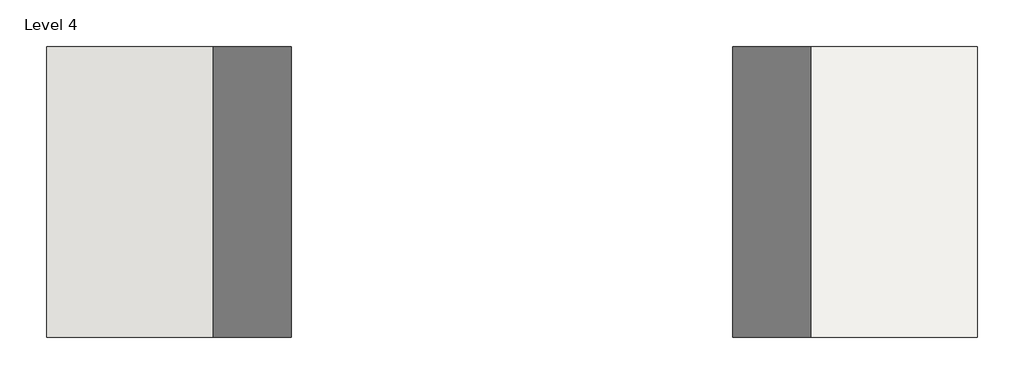
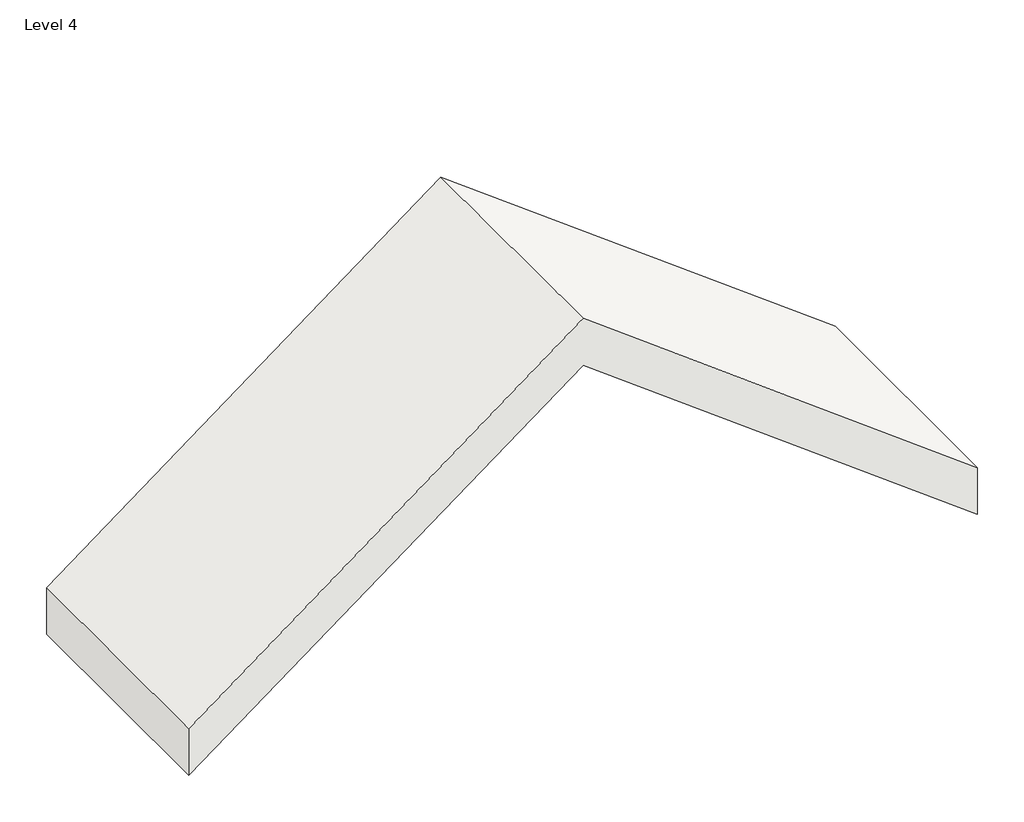
# One storey: 1 roof.
"""IFC4 building model written with IfcOpenShell, lengths in millimetres."""

from ifc_helpers import new_model, si_unit, frame, origin, place, context, project, spatial, polyline, outline, extrude, element, save

model = new_model("IFC4")

# Units and contexts
model_context = context("Model", 3, world=origin())
ifc_project = project(units=[si_unit("LENGTHUNIT", "METRE", prefix="MILLI")], contexts=[model_context])

# Site, building, storey
site = spatial("IfcSite", under=ifc_project)
building = spatial("IfcBuilding", under=site)
storey = spatial("IfcBuildingStorey", under=building, Name="Level 4", Elevation=9144.0)

# Roof
placement = place(None, origin())
element("IfcRoof", 1, ObjectType="Generic - 12\"", at=placement, inside=storey, context=model_context, shape_type="SweptSolid", body=[
    extrude(outline(polyline([(9525.0, -10404.6498106), (11809.2644938, -13450.3358024), (9525.0, -16496.0217941), (9144.0, -16496.0217941), (11428.2644938, -13450.3358024), (9144.0, -10404.6498106), (9525.0, -10404.6498106)])), frame((0.0, -12865.0511954, 0.0), z_axis=(0.0, 1.0, 0.0), x_axis=(0.0, 0.0, 1.0)), (0.0, 0.0, 1.0), 1901.825),
])

save(model, "model.ifc")

# Revit data of these elements
# Type "Generic - 12\""
#   Assembly Code = "B1020"
#   Layers, outside or top first: 1' - 0" no material (function 1)
# Element 1 (IfcRoof, "Generic - 12\"")
#   built-in parameter 1001705 = 38.7443 (stored number, unit not read)
#   built-in parameter 1001710 = 33615
#   Phase Created = New Construction
#   Materials on its faces: "Default Roof"
# Materials
#   "Default Roof": colour RGB 88 101 114, transparency 0, Cost = 0
